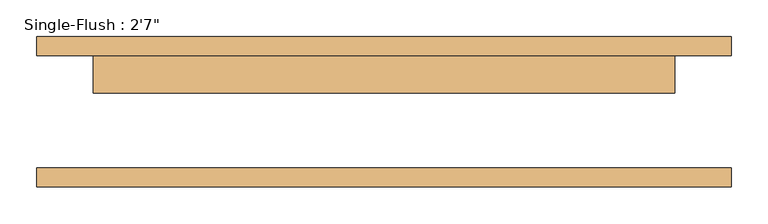
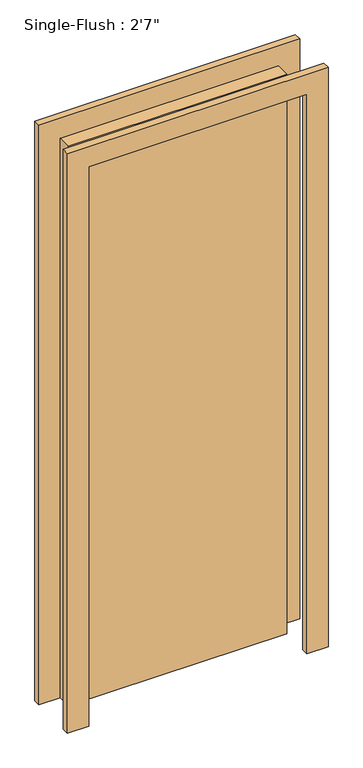
"""IFC4 building model written with IfcOpenShell, lengths in millimetres: door geometry."""

from ifc_helpers import new_model, si_unit, frame, origin, origin_with_axes, place, context, project, spatial, polyline, outline, extrude, source, transform, mapped, element, save


def door_b804d09e(model_context):
    return source(origin(), model_context, "Body", "SweptSolid", [
        extrude(outline(polyline([(2209.8, -469.9), (0.0, -469.9), (0.0, -393.7), (2133.6, -393.7), (2133.6, 393.7), (0.0, 393.7), (0.0, 469.9), (2209.8, 469.9), (2209.8, -469.9)])), frame((0.0, 76.2, 0.0), z_axis=(0.0, 1.0, 0.0), x_axis=(0.0, 0.0, 1.0)), (0.0, 0.0, 1.0), 25.4),
        extrude(outline(polyline([(2209.8, 469.9), (2209.8, -469.9), (0.0, -469.9), (0.0, -393.7), (2133.6, -393.7), (2133.6, 393.7), (0.0, 393.7), (0.0, 469.9), (2209.8, 469.9)])), frame((0.0, -101.6, 0.0), z_axis=(0.0, 1.0, 0.0), x_axis=(0.0, 0.0, 1.0)), (0.0, 0.0, 1.0), 25.4),
        extrude(outline(polyline([(393.7, 25.4), (-393.7, 25.4), (-393.7, 76.2), (393.7, 76.2), (393.7, 25.4)])), origin_with_axes(), (0.0, 0.0, 1.0), 2133.6),
    ])


if __name__ == "__main__":
    model = new_model("IFC4")
    model_context = context("Model", 3, world=origin())
    ifc_project = project(units=[si_unit("LENGTHUNIT", "METRE", prefix="MILLI")], contexts=[model_context])
    site = spatial("IfcSite", under=ifc_project)
    building = spatial("IfcBuilding", under=site)
    placement = place(None, origin())
    door_shape = door_b804d09e(model_context)
    element("IfcDoor", 1, ObjectType="Single-Flush : 2'7\"", at=placement, inside=building, context=model_context, shape_type="MappedRepresentation", body=[
        mapped(door_shape, transform((0.0, 0.0, 0.0), x_axis=(1.0, 0.0, 0.0), y_axis=(0.0, 1.0, 0.0), z_axis=(0.0, 0.0, 1.0))),
    ])
    save(model, "model.ifc")

# Revit data of these elements
# Type "Single-Flush : 2'7\""
#   Type Mark = "8"
#   Construction Type Id = "MDOOR"
#   Assembly Code = "C1020"
#   Analytic Construction = "Metal"
#   Thickness = 0' - 2"
#   Heat Transfer Coefficient (U) = 0.651978 BTU/(h·ft²·°F)
#   Height = 7' - 0"
#   Trim Projection Ext = 0' - 1"
#   Trim Projection Int = 0' - 1"
#   Trim Width = 0' - 3"
#   Width = 2' - 7"
#   Define Thermal Properties by = 1
#   Door Material = Door - Panel
#   Frame Material = Door - Frame
#   Visual Light Transmittance = 0
#   Solar Heat Gain Coefficient = 0
#   Function = (empty or 0)
#   Wall Closure = (empty or 0)
# Element 1 (IfcDoor, "Single-Flush : 2'7\"")
#   Materials on its faces: "Door - Frame", "Door - Panel"
# Materials
#   "Door - Panel": class "Wood", colour RGB 210 159 95, transparency 0
#   "Door - Frame": colour RGB 118 70 51, transparency 0
